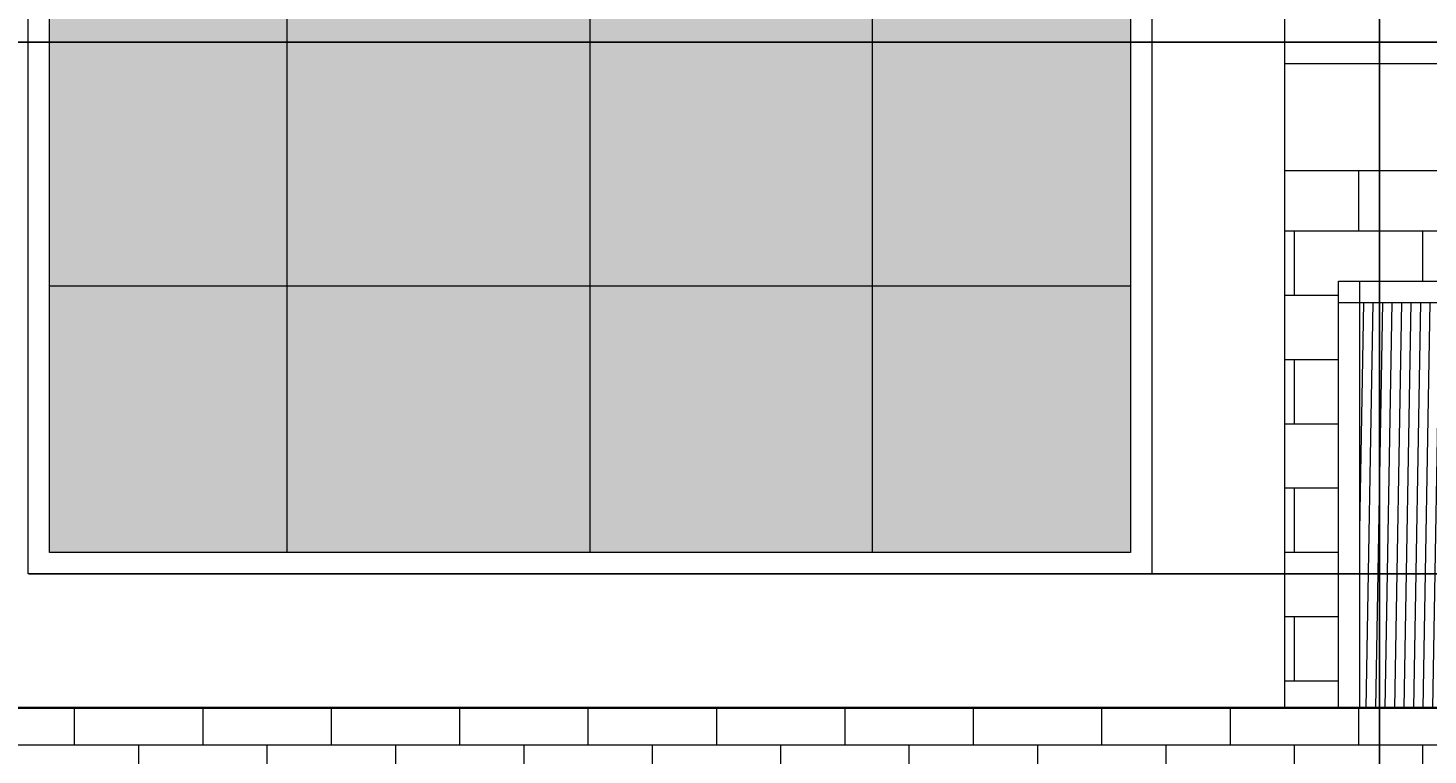
# Model space of a CAD drawing. Units: inches. Extents: x -26 to 776, y -22 to 650.
# Tile 9 of 62: x 92 to 222, y 155 to 223. Entities that reach past the tile are written whole.
import ezdxf

# ---------------------------------------------------------------- set-up
doc = ezdxf.new("R2010")
doc.units = ezdxf.units.IN
doc.header["$MEASUREMENT"] = 0
for name, color, linetype, lineweight in [('A-ANNO-DIMS', 2, 'Continuous', 18), ('A-DETL-PATT', 8, 'Continuous', 13), ('A-GLAZ', 4, 'Continuous', 18), ('A-GLAZ-PATT', 9, 'Continuous', 13), ('A-WALL', 7, 'Continuous', 35), ('A-WALL-PATT', 8, 'Continuous', 13), ('A-WALL-TRIM', 7, 'Continuous', 18)]:
    doc.layers.add(name, color=color, linetype=linetype, lineweight=lineweight)
doc.styles.get("Standard").update_dxf_attribs({"font": 'arial.ttf'})
doc.dimstyles.get("Standard").update_dxf_attribs({"dimtxt": 0.5625, "dimasz": 0.18, "dimexe": 0.18, "dimexo": 0.0625, "dimgap": 0.09, "dimtad": 0, "dimtih": 1, "dimtoh": 1, "dimdec": 4, "dimzin": 0, "dimdsep": 46, "dimlunit": 4, "dimtxsty": 'Standard', "dimcen": 0.09, "dimadec": 0, "dimazin": 0, "dimtfac": 1, "dimtdec": 4, "dimtofl": 0, "dimtmove": 0, "dimatfit": 3, "dimfxl": 1, "dimtolj": 1, "dimtzin": 0, "dimarcsym": 0})

# ---------------------------------------------------------------- blocks, each defined once
blk = doc.blocks.new('WIN-ELEV-4X4')
for p, q in [((24.2, 97.34), (24.2, 2)), ((52.51, 97.34), (52.51, 2)), ((78.9, 97.34), (78.9, 2)), ((2, 76.47), (103.02, 76.47)), ((2, 76.47), (103.02, 76.47)), ((2, 52.37), (103.02, 52.37)), ((2, 26.9), (103.02, 26.9))]:
    blk.add_line(p, q)
for points in [[(0, 99.34), (105.02, 99.34), (105.02, 0), (0, 0)], [(2, 97.34), (103.02, 97.34), (103.02, 2), (2, 2)]]:
    blk.add_lwpolyline(points, close=True)
blk = doc.blocks.new('*D14')
at = {"layer": 'A-ANNO-DIMS', "color": 0, "lineweight": -2, "transparency": 16777216}
for p, q in [((191.62, 613.27), (-25.48, 613.27)), ((-25.3, 613.09), (-25.3, 314.75)), ((-25.3, 15.66), (-25.3, 314)), ((11.04, 15.48), (-25.48, 15.48))]:
    blk.add_line(p, q, dxfattribs=at)
at = {"layer": 'A-ANNO-DIMS', "color": 0, "transparency": 16777216}
for points in [[(-25.33, 613.09), (-25.27, 613.09), (-25.3, 613.27)], [(-25.33, 15.66), (-25.27, 15.66), (-25.3, 15.48)]]:
    blk.add_solid(points, dxfattribs=at)
at = {"layer": 'Defpoints', "color": 0, "transparency": 16777216}
for p in [(-25.3, 613.27), (191.68, 613.27), (11.11, 15.48)]:
    blk.add_point(p, dxfattribs=at)
at = {"layer": 'A-ANNO-DIMS', "color": 0, "transparency": 16777216, "insert": (-25.3, 314.38), "char_height": 0.562, "attachment_point": 5}
blk.add_mtext('\\A1;597.8', dxfattribs=at)
blk = doc.blocks.new('*D22')
at = {"layer": 'A-ANNO-DIMS', "color": 0, "lineweight": -2, "transparency": 16777216}
for p, q in [((22.89, 15.33), (22.89, 649.86)), ((23.07, 649.68), (119.19, 649.68)), ((217.77, 649.68), (121.65, 649.68)), ((217.95, 15.54), (217.95, 649.86))]:
    blk.add_line(p, q, dxfattribs=at)
at = {"layer": 'A-ANNO-DIMS', "color": 0, "transparency": 16777216}
for points in [[(23.07, 649.71), (23.07, 649.65), (22.89, 649.68)], [(217.77, 649.71), (217.77, 649.65), (217.95, 649.68)]]:
    blk.add_solid(points, dxfattribs=at)
at = {"layer": 'Defpoints', "color": 0, "transparency": 16777216}
for p in [(217.95, 649.68), (22.89, 15.27), (217.95, 15.48)]:
    blk.add_point(p, dxfattribs=at)
at = {"layer": 'A-ANNO-DIMS', "color": 0, "transparency": 16777216, "insert": (120.42, 649.68), "char_height": 0.562, "attachment_point": 5}
blk.add_mtext('\\A1;195.06', dxfattribs=at)
blk = doc.blocks.new('*D26')
at = {"layer": 'A-ANNO-DIMS', "color": 0, "lineweight": -2, "transparency": 16777216}
for p, q in [((91.71, 171.97), (775.34, 171.97)), ((775.16, 171.79), (775.16, 166.11)), ((775.16, 159.66), (775.16, 165.35)), ((82.2, 159.48), (775.34, 159.48))]:
    blk.add_line(p, q, dxfattribs=at)
at = {"layer": 'A-ANNO-DIMS', "color": 0, "transparency": 16777216}
for points in [[(775.13, 171.79), (775.19, 171.79), (775.16, 171.97)], [(775.13, 159.66), (775.19, 159.66), (775.16, 159.48)]]:
    blk.add_solid(points, dxfattribs=at)
at = {"layer": 'Defpoints', "color": 0, "transparency": 16777216}
for p in [(91.64, 171.97), (775.16, 171.97), (82.13, 159.48)]:
    blk.add_point(p, dxfattribs=at)
at = {"layer": 'A-ANNO-DIMS', "color": 0, "transparency": 16777216, "insert": (775.16, 165.73), "char_height": 0.562, "attachment_point": 5}
blk.add_mtext('\\A1;12.49', dxfattribs=at)
blk = doc.blocks.new('*D37')
at = {"layer": 'A-ANNO-DIMS', "color": 0, "lineweight": -2, "transparency": 16777216}
for p, q in [((231.36, 159.48), (-25.48, 159.48)), ((-25.3, 159.3), (-25.3, 87.85)), ((-25.3, 15.66), (-25.3, 87.11)), ((217.89, 15.48), (-25.48, 15.48))]:
    blk.add_line(p, q, dxfattribs=at)
at = {"layer": 'A-ANNO-DIMS', "color": 0, "transparency": 16777216}
for points in [[(-25.33, 159.3), (-25.27, 159.3), (-25.3, 159.48)], [(-25.33, 15.66), (-25.27, 15.66), (-25.3, 15.48)]]:
    blk.add_solid(points, dxfattribs=at)
at = {"layer": 'Defpoints', "color": 0, "transparency": 16777216}
for p in [(-25.3, 159.48), (231.42, 159.48), (217.95, 15.48)]:
    blk.add_point(p, dxfattribs=at)
at = {"layer": 'A-ANNO-DIMS', "color": 0, "transparency": 16777216, "insert": (-25.3, 87.48), "char_height": 0.562, "attachment_point": 5}
blk.add_mtext('\\A1;144', dxfattribs=at)
blk = doc.blocks.new('*D41')
at = {"layer": 'A-ANNO-DIMS', "color": 0, "lineweight": -2, "transparency": 16777216}
for p, q in [((11.17, 221.64), (775.34, 221.64)), ((775.16, 221.46), (775.16, 190.94)), ((775.16, 159.66), (775.16, 190.18)), ((11.17, 159.48), (775.34, 159.48))]:
    blk.add_line(p, q, dxfattribs=at)
at = {"layer": 'A-ANNO-DIMS', "color": 0, "transparency": 16777216}
for points in [[(775.13, 221.46), (775.19, 221.46), (775.16, 221.64)], [(775.13, 159.66), (775.19, 159.66), (775.16, 159.48)]]:
    blk.add_solid(points, dxfattribs=at)
at = {"layer": 'Defpoints', "color": 0, "transparency": 16777216}
for p in [(11.11, 221.64), (775.16, 221.64), (11.11, 159.48)]:
    blk.add_point(p, dxfattribs=at)
at = {"layer": 'A-ANNO-DIMS', "color": 0, "transparency": 16777216, "insert": (775.16, 190.56), "char_height": 0.562, "attachment_point": 5}
blk.add_mtext('\\A1;62.16', dxfattribs=at)

msp = doc.modelspace()

# ---------------------------------------------------------------- hatches: boundary and pattern name
at = {"layer": 'A-DETL-PATT'}
h = msp.add_hatch(dxfattribs=at)
h.set_pattern_fill('ANSI31', color=256, scale=7.1, angle=44)
h.paths.add_polyline_path([(231.4249, 197.3298), (216.1056, 197.3298), (216.1056, 159.4824), (231.4249, 159.4824)])
h.paths.add_polyline_path([(236.4647, 197.3298), (231.4249, 197.3298), (231.4249, 159.4824), (276.1134, 159.4824), (276.1134, 171.4173), (236.4647, 171.4173)])
h.paths.add_polyline_path([(259.7413, 197.3298), (236.4647, 197.3298), (236.4647, 171.4173), (259.7413, 171.4173)], flags=17)
h.paths.add_polyline_path([(276.1134, 197.3298), (261.7413, 197.3298), (261.7413, 171.4173), (276.1134, 171.4173)], flags=17)
h.paths.add_polyline_path([(217.9529, 147.0781), (22.8891, 147.0781), (22.8891, 138.3844), (217.9529, 138.3844)])
h.paths.add_polyline_path([(285.0179, 152.3087), (285.0179, 159.4824), (231.4249, 159.4824), (240.1654, 144.8359), (280.6173, 144.8359)])
h.paths.add_polyline_path([(280.6173, 144.8359), (240.1654, 144.8359), (240.1654, 26.4239), (280.6173, 26.4239)])
h.paths.add_polyline_path([(274.6644, 134.8811), (274.6644, 34.0885), (245.7207, 34.0885), (245.7207, 134.8811)], flags=16)
h.paths.add_polyline_path([(285.0179, 303.3046), (236.4647, 303.3046), (236.4647, 294.4171), (285.0179, 294.4171)])
h.paths.add_polyline_path([(285.0179, 446.0063), (236.4647, 446.0063), (236.4647, 437.1188), (285.0179, 437.1188)])
at = {"layer": 'A-GLAZ-PATT'}
h = msp.add_hatch(dxfattribs=at)
h.set_pattern_fill('GOST_GLASS', color=256, scale=0.75)
h.set_pattern_definition([(45, (0, 0), (6.36396, 0), [3.75, -5.25]), (45, (1.591, 0), (6.36396, 0), [1.5, -7.5]), (45, (0, 1.591), (6.36396, 0), [1.5, -7.5])])
h.paths.add_polyline_path([(115.8402, 198.8773), (93.6448, 198.8773), (93.6448, 173.9734), (115.8402, 173.9734)])
h.paths.add_polyline_path([(144.1571, 198.8773), (115.8402, 198.8773), (115.8402, 173.9734), (144.1571, 173.9734)])
h.paths.add_polyline_path([(115.8402, 224.3396), (93.6448, 224.3396), (93.6448, 198.8773), (115.8402, 198.8773)])
h.paths.add_polyline_path([(144.1571, 248.4417), (115.8402, 248.4417), (115.8402, 224.3396), (144.1571, 224.3396)])
h.paths.add_polyline_path([(144.1571, 224.3396), (115.8402, 224.3396), (115.8402, 198.8773), (144.1571, 198.8773)])
h.paths.add_polyline_path([(170.5449, 224.3396), (144.1571, 224.3396), (144.1571, 198.8773), (170.5449, 198.8773)])
h.paths.add_polyline_path([(170.5449, 198.8773), (144.1571, 198.8773), (144.1571, 173.9734), (170.5449, 173.9734)])
h.paths.add_polyline_path([(194.6694, 198.8773), (170.5449, 198.8773), (170.5449, 173.9734), (194.6694, 173.9734)])
h.paths.add_polyline_path([(194.6694, 224.3396), (170.5449, 224.3396), (170.5449, 198.8773), (194.6694, 198.8773)])
h.paths.add_polyline_path([(194.6694, 248.4417), (170.5449, 248.4417), (170.5449, 224.3396), (194.6694, 224.3396)])
h.paths.add_polyline_path([(170.5449, 248.4417), (144.1571, 248.4417), (144.1571, 224.3396), (170.5449, 224.3396)])
h.paths.add_polyline_path([(144.1571, 269.3091), (115.8402, 269.3091), (115.8402, 248.4417), (144.1571, 248.4417)])
h.paths.add_polyline_path([(115.8402, 269.3091), (93.6448, 269.3091), (93.6448, 248.4417), (115.8402, 248.4417)])
h.paths.add_polyline_path([(115.8402, 248.4417), (93.6448, 248.4417), (93.6448, 224.3396), (115.8402, 224.3396)])
h.paths.add_polyline_path([(170.5449, 269.3091), (144.1571, 269.3091), (144.1571, 248.4417), (170.5449, 248.4417)])
h.paths.add_polyline_path([(194.6694, 269.3091), (170.5449, 269.3091), (170.5449, 248.4417), (194.6694, 248.4417)])
h.paths.add_polyline_path([(259.7413, 294.4171), (236.4647, 294.4171), (236.4647, 266.1888), (259.7413, 266.1888)])
h.paths.add_polyline_path([(285.0179, 294.4171), (261.7413, 294.4171), (261.7413, 266.1888), (285.0179, 266.1888)])
h.paths.add_polyline_path([(285.0179, 265.1888), (261.7413, 265.1888), (261.7413, 233.9172), (285.0179, 233.9172)])
h.paths.add_polyline_path([(259.7413, 265.1888), (236.4647, 265.1888), (236.4647, 233.9172), (259.7413, 233.9172)])
h.paths.add_polyline_path([(259.7413, 232.9172), (236.4647, 232.9172), (236.4647, 207.1741), (259.7413, 207.1741)])
h.paths.add_polyline_path([(285.0179, 232.9172), (261.7413, 232.9172), (261.7413, 207.1741), (285.0179, 207.1741)])
h.paths.add_polyline_path([(285.0179, 206.1741), (261.7413, 206.1741), (261.7413, 199.3298), (278.1134, 199.3298), (278.1134, 171.4173), (285.0179, 171.4173)])
h.paths.add_polyline_path([(259.7413, 206.1741), (236.4647, 206.1741), (236.4647, 199.3298), (259.7413, 199.3298)])
h.paths.add_polyline_path([(259.7413, 197.3298), (236.4647, 197.3298), (236.4647, 171.4173), (259.7413, 171.4173)])
h.paths.add_polyline_path([(276.1134, 197.3298), (261.7413, 197.3298), (261.7413, 171.4173), (276.1134, 171.4173)], flags=17)
h.paths.add_polyline_path([(255.8125, 548.0348), (228.5733, 548.0348), (228.5733, 528.3585), (255.8125, 528.3585)])
h.paths.add_polyline_path([(281.6181, 548.0348), (256.0792, 548.0348), (256.0792, 528.3585), (281.6181, 528.3585)])
h.paths.add_polyline_path([(308.8797, 548.0348), (281.789, 548.0348), (281.789, 528.3585), (308.8797, 528.3585)])
h.paths.add_polyline_path([(357.2724, 548.0995), (309.2457, 548.0348), (309.2457, 528.3585), (357.3034, 528.4233), (357.3034, 538.2614)])
h.paths.add_polyline_path([(259.7413, 437.1188), (236.4647, 437.1188), (236.4647, 408.8905), (259.7413, 408.8905)])
h.paths.add_polyline_path([(285.0179, 437.1188), (261.7413, 437.1188), (261.7413, 408.8905), (285.0179, 408.8905)])
h.paths.add_polyline_path([(259.7413, 407.8905), (236.4647, 407.8905), (236.4647, 376.6189), (259.7413, 376.6189)])
h.paths.add_polyline_path([(285.0179, 407.8905), (261.7413, 407.8905), (261.7413, 376.6189), (285.0179, 376.6189)])
h.paths.add_polyline_path([(285.0179, 375.6189), (261.7413, 375.6189), (261.7413, 349.8758), (285.0179, 349.8758)])
h.paths.add_polyline_path([(285.0179, 348.8758), (261.7413, 348.8758), (261.7413, 314.119), (285.0179, 314.119)])
h.paths.add_polyline_path([(259.7413, 348.8758), (236.4647, 348.8758), (236.4647, 314.119), (259.7413, 314.119)])
h.paths.add_polyline_path([(259.7413, 375.6189), (236.4647, 375.6189), (236.4647, 349.8758), (259.7413, 349.8758)])
h.paths.add_polyline_path([(194.6694, 404.1909), (170.5449, 404.1909), (170.5449, 383.3235), (194.6694, 383.3235)])
h.paths.add_polyline_path([(170.5449, 404.1909), (144.1571, 404.1909), (144.1571, 383.3235), (170.5449, 383.3235)])
h.paths.add_polyline_path([(144.1571, 404.1909), (115.8402, 404.1909), (115.8402, 383.3235), (144.1571, 383.3235)])
h.paths.add_polyline_path([(115.8402, 404.1909), (93.6448, 404.1909), (93.6448, 383.3235), (115.8402, 383.3235)])
h.paths.add_polyline_path([(115.8402, 383.3235), (93.6448, 383.3235), (93.6448, 359.2214), (115.8402, 359.2214)])
h.paths.add_polyline_path([(144.1571, 383.3235), (115.8402, 383.3235), (115.8402, 359.2214), (144.1571, 359.2214)])
h.paths.add_polyline_path([(115.8402, 359.2214), (93.6448, 359.2214), (93.6448, 333.7591), (115.8402, 333.7591)])
h.paths.add_polyline_path([(144.1571, 359.2214), (115.8402, 359.2214), (115.8402, 333.7591), (144.1571, 333.7591)])
h.paths.add_polyline_path([(115.8402, 333.7591), (93.6448, 333.7591), (93.6448, 308.8552), (115.8402, 308.8552)])
h.paths.add_polyline_path([(144.1571, 333.7591), (115.8402, 333.7591), (115.8402, 308.8552), (144.1571, 308.8552)])
h.paths.add_polyline_path([(170.5449, 333.7591), (144.1571, 333.7591), (144.1571, 308.8552), (170.5449, 308.8552)])
h.paths.add_polyline_path([(170.5449, 359.2214), (144.1571, 359.2214), (144.1571, 333.7591), (170.5449, 333.7591)])
h.paths.add_polyline_path([(170.5449, 383.3235), (144.1571, 383.3235), (144.1571, 359.2214), (170.5449, 359.2214)])
h.paths.add_polyline_path([(194.6694, 383.3235), (170.5449, 383.3235), (170.5449, 359.2214), (194.6694, 359.2214)])
h.paths.add_polyline_path([(194.6694, 359.2214), (170.5449, 359.2214), (170.5449, 333.7591), (194.6694, 333.7591)])
h.paths.add_polyline_path([(194.6694, 333.7591), (170.5449, 333.7591), (170.5449, 308.8552), (194.6694, 308.8552)])
at = {"layer": 'A-WALL-PATT'}
h = msp.add_hatch(dxfattribs=at)
h.set_pattern_fill('AR-B816', color=256, scale=0.75)
h.paths.add_polyline_path([(82.134, 209.6413), (11.1074, 209.6413), (11.1074, 159.4824), (82.134, 159.4824)])
h.paths.add_polyline_path([(231.4249, 209.6413), (209.091, 209.6413), (209.091, 159.4824), (214.1056, 159.4824), (214.1056, 199.3298), (231.4249, 199.3298)])
h.paths.add_polyline_path([(231.4249, 159.4824), (11.1074, 159.4824), (11.1074, 22.5014), (22.8891, 22.5014), (22.8891, 147.0781), (217.9529, 147.0781), (217.9529, 20.7937), (231.4249, 20.7937)])
h.paths.add_polyline_path([(285.0179, 152.3087), (280.6173, 144.8359), (280.6173, 26.4239), (240.1654, 26.4239), (240.1654, 144.8359), (231.4249, 159.4824), (231.4249, 20.7937), (285.0179, 20.7937)])

# ---------------------------------------------------------------- linework, layer by layer
at = {"layer": 'A-WALL'}
msp.add_line((11.1074, 159.4824), (231.4249, 159.4824), dxfattribs=at)
at = {"layer": 'A-WALL-TRIM'}
for p, q in [((209.091, 221.6413), (231.4249, 221.6413)), ((209.091, 219.6413), (231.4249, 219.6413)), ((209.091, 209.6413), (231.4249, 209.6413)), ((214.1056, 159.4824), (214.1056, 199.3298)), ((214.1056, 199.3298), (278.1134, 199.3298)), ((216.1056, 159.4824), (216.1056, 199.3298)), ((214.1056, 197.3298), (278.1134, 197.3298))]:
    msp.add_line(p, q, dxfattribs=at)
msp.add_lwpolyline([(82.134, 159.4824), (209.091, 159.4824), (209.091, 420.2783), (82.134, 420.2783)], close=True, dxfattribs=at)

# ---------------------------------------------------------------- block references
at = {"layer": 'A-GLAZ'}
msp.add_blockref('WIN-ELEV-4X4', (91.645, 171.9733), dxfattribs=at)

# ---------------------------------------------------------------- dimensions: what is measured, and where the dimension line sits
at = {"layer": 'A-ANNO-DIMS'}
dim = msp.add_linear_dim(base=(217.9529, 649.6763), p1=(22.8891, 15.2701), p2=(217.9529, 15.4824), dimstyle='Standard', override={"dimdec": 2, "dimlfac": 1, "dimrnd": 0, "dimzin": 0, "dimdsep": 46, "dimlunit": 2}, dxfattribs=at)
dim.commit()
dim.dimension.update_dxf_attribs({"geometry": '*D22', "text_midpoint": (120.421, 649.6763)})
for base, p1, p2, override, picture, middle in [((-25.2976, 613.2713), (11.1074, 15.4824), (191.6782, 613.2713), {"dimdec": 1, "dimlfac": 1, "dimrnd": 0, "dimzin": 0, "dimdsep": 46, "dimlunit": 2}, '*D14', (-25.2976, 314.3769)), ((775.1553, 221.6413), (11.1074, 159.4824), (11.1074, 221.6413), {"dimdec": 2, "dimlfac": 1, "dimrnd": 0, "dimzin": 0, "dimdsep": 46, "dimlunit": 2}, '*D41', (775.1553, 190.5618)), ((775.1553, 171.9734), (82.134, 159.4824), (91.6448, 171.9734), {"dimdec": 2, "dimlfac": 1, "dimrnd": 0, "dimzin": 0, "dimdsep": 46, "dimlunit": 2}, '*D26', (775.1553, 165.7279)), ((-25.2976, 159.4824), (217.9529, 15.4824), (231.4249, 159.4824), {"dimdec": 0, "dimlfac": 1, "dimrnd": 0, "dimzin": 0, "dimdsep": 46, "dimlunit": 2}, '*D37', (-25.2976, 87.4824))]:
    dim = msp.add_linear_dim(base=base, p1=p1, p2=p2, angle=90, dimstyle='Standard', override=override, dxfattribs=at)
    dim.commit()
    dim.dimension.update_dxf_attribs({"geometry": picture, "text_midpoint": middle})

doc.saveas('drawing.dxf')
